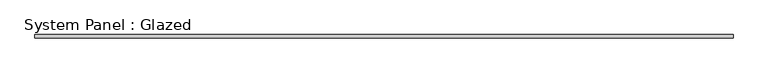
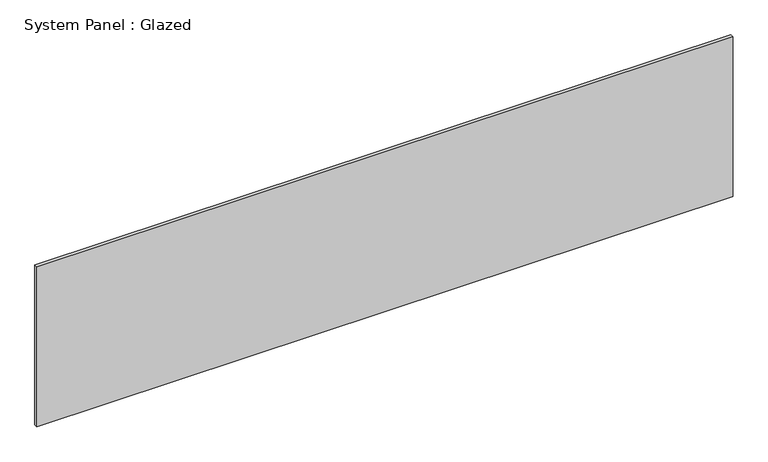
"""IFC4 building model written with IfcOpenShell, lengths in millimetres: plate geometry, System Panel : Glazed."""

from ifc_helpers import new_model, si_unit, origin, origin_with_axes, place, context, project, spatial, polyline, outline, extrude, source, transform, mapped, element, save


def system_panel_glazed_a5f349e9(model_context):
    return source(origin(), model_context, "Body", "SweptSolid", [
        extrude(outline(polyline([(2511.425, 19.05), (-2511.425, 19.05), (-2511.425, 44.45), (2511.425, 44.45), (2511.425, 19.05)])), origin_with_axes(), (0.0, 0.0, 1.0), 1219.2),
    ])


if __name__ == "__main__":
    model = new_model("IFC4")
    model_context = context("Model", 3, world=origin())
    ifc_project = project(units=[si_unit("LENGTHUNIT", "METRE", prefix="MILLI")], contexts=[model_context])
    site = spatial("IfcSite", under=ifc_project)
    building = spatial("IfcBuilding", under=site)
    placement = place(None, origin())
    system_panel_glazed_shape = system_panel_glazed_a5f349e9(model_context)
    element("IfcPlate", 1, ObjectType="System Panel : Glazed", at=placement, inside=building, context=model_context, shape_type="MappedRepresentation", body=[
        mapped(system_panel_glazed_shape, transform((0.0, 0.0, 0.0), x_axis=(1.0, 0.0, 0.0), y_axis=(0.0, 1.0, 0.0), z_axis=(0.0, 0.0, 1.0))),
    ])
    save(model, "model.ifc")

# Revit data of these elements
# Type "System Panel : Glazed"
#   Construction Type Id = "GSP4R"
#   Analytic Construction = "1/8 in Pilkington single glazing"
#   Visual Light Transmittance = 0.9
#   Solar Heat Gain Coefficient = 0.86
#   Heat Transfer Coefficient (U) = 1.18115 BTU/(h·ft²·°F)
# Element 1 (IfcPlate, "System Panel : Glazed")
#   Materials on its faces: "Glass"
# Materials
#   "Glass": class "Glass", colour RGB 0 128 192, transparency 0.75, Description = "Soda Lime Glass", Cost = 0
